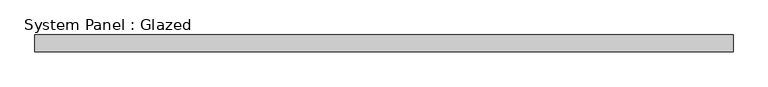
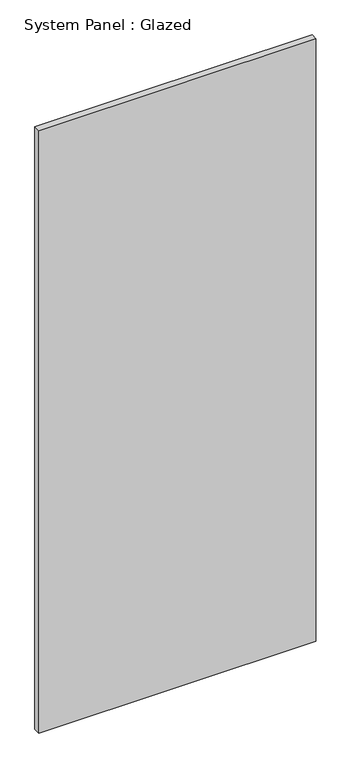
"""IFC4 building model written with IfcOpenShell, lengths in millimetres: plate geometry, System Panel : Glazed."""

from ifc_helpers import new_model, si_unit, origin, origin_with_axes, place, context, project, spatial, polyline, outline, extrude, source, transform, mapped, element, save


def system_panel_glazed_4603f3ec(model_context):
    return source(origin(), model_context, "Body", "SweptSolid", [
        extrude(outline(polyline([(522.2400148, 24.5), (-522.2400148, 24.5), (-522.2400148, 49.5), (522.2400148, 49.5), (522.2400148, 24.5)])), origin_with_axes(), (0.0, 0.0, 1.0), 2400.0242188),
    ])


if __name__ == "__main__":
    model = new_model("IFC4")
    model_context = context("Model", 3, world=origin())
    ifc_project = project(units=[si_unit("LENGTHUNIT", "METRE", prefix="MILLI")], contexts=[model_context])
    site = spatial("IfcSite", under=ifc_project)
    building = spatial("IfcBuilding", under=site)
    placement = place(None, origin())
    system_panel_glazed_shape = system_panel_glazed_4603f3ec(model_context)
    element("IfcPlate", 1, ObjectType="System Panel : Glazed", at=placement, inside=building, context=model_context, shape_type="MappedRepresentation", body=[
        mapped(system_panel_glazed_shape, transform((0.0, 0.0, 0.0), x_axis=(1.0, 0.0, 0.0), y_axis=(0.0, 1.0, 0.0), z_axis=(0.0, 0.0, 1.0))),
    ])
    save(model, "model.ifc")

# Revit data of these elements
# Type "System Panel : Glazed"
#   Keynote = "H11"
#   Construction Type Id = "GSP4R"
#   Analytic Construction = "1/8 in Pilkington single glazing"
#   Visual Light Transmittance = 0.9
#   Solar Heat Gain Coefficient = 0.86
#   Heat Transfer Coefficient (U) = 6.7069 W/(m²·K)
#   Define Thermal Properties by = 1
# Element 1 (IfcPlate, "System Panel : Glazed")
#   Materials on its faces: "Glass"
# Materials
#   "Glass": class "Glass", colour RGB 0 128 192, transparency 0.9, Description = "Soda Lime Glass", Cost = 0
